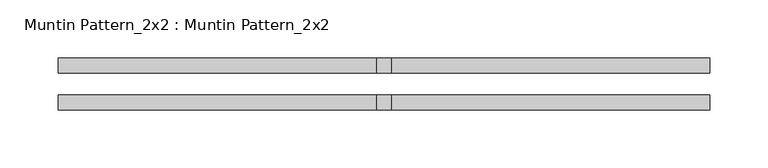
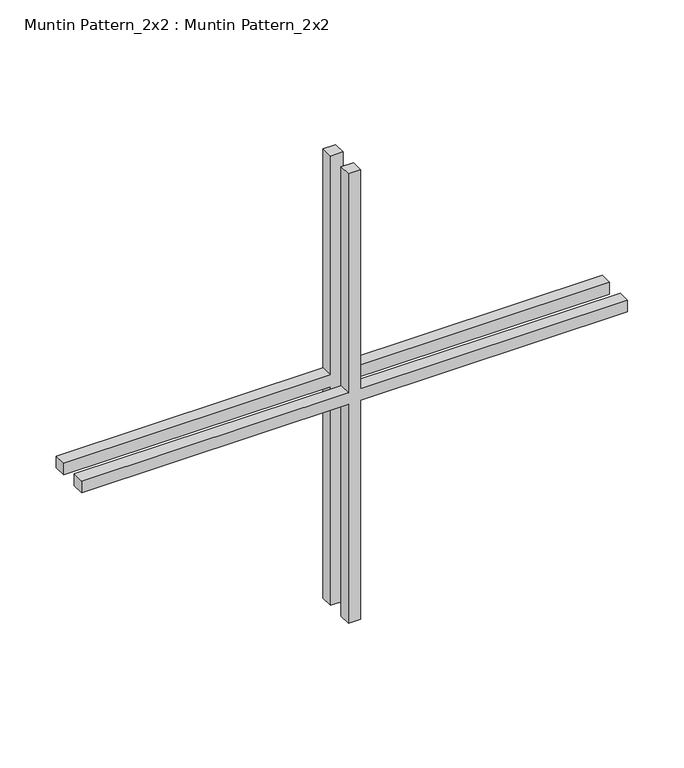
"""IFC4 building model written with IfcOpenShell, lengths in millimetres: proxy geometry, Muntin Pattern_2x2 : Muntin Pattern_2x2."""

from ifc_helpers import new_model, si_unit, frame, origin, place, context, project, spatial, polyline, outline, extrude, source, transform, mapped, element, save


def muntin_pattern_2x2_muntin_pattern_2x2_5f474966(model_context):
    return source(origin(), model_context, "Body", "SweptSolid", [
        extrude(outline(polyline([(249.2375, -6.35), (249.2375, -279.4), (236.5375, -279.4), (236.5375, -6.35), (0.0, -6.35), (0.0, 6.35), (236.5375, 6.35), (236.5375, 279.4), (249.2375, 279.4), (249.2375, 6.35), (485.775, 6.35), (485.775, -6.35), (249.2375, -6.35)])), frame((0.0, 9.525, 0.0), z_axis=(0.0, 1.0, 0.0), x_axis=(0.0, 0.0, 1.0)), (0.0, 0.0, 1.0), 12.7),
        extrude(outline(polyline([(249.2375, -6.35), (249.2375, -279.4), (236.5375, -279.4), (236.5375, -6.35), (0.0, -6.35), (0.0, 6.35), (236.5375, 6.35), (236.5375, 279.4), (249.2375, 279.4), (249.2375, 6.35), (485.775, 6.35), (485.775, -6.35), (249.2375, -6.35)])), frame((0.0, -22.225, 0.0), z_axis=(0.0, 1.0, 0.0), x_axis=(0.0, 0.0, 1.0)), (0.0, 0.0, 1.0), 12.7),
    ])


if __name__ == "__main__":
    model = new_model("IFC4")
    model_context = context("Model", 3, world=origin())
    ifc_project = project(units=[si_unit("LENGTHUNIT", "METRE", prefix="MILLI")], contexts=[model_context])
    site = spatial("IfcSite", under=ifc_project)
    building = spatial("IfcBuilding", under=site)
    placement = place(None, origin())
    muntin_pattern_2x2_muntin_pattern_2x2_shape = muntin_pattern_2x2_muntin_pattern_2x2_5f474966(model_context)
    element("IfcBuildingElementProxy", 1, Name="Muntin Pattern_2x2 : Muntin Pattern_2x2", ObjectType="Muntin Pattern_2x2 : Muntin Pattern_2x2", at=placement, inside=building, context=model_context, shape_type="MappedRepresentation", body=[
        mapped(muntin_pattern_2x2_muntin_pattern_2x2_shape, transform((0.0, 0.0, 0.0), x_axis=(1.0, 0.0, 0.0), y_axis=(0.0, 1.0, 0.0), z_axis=(0.0, 0.0, 1.0))),
    ])
    save(model, "model.ifc")

# Revit data of these elements
# Type "Muntin Pattern_2x2 : Muntin Pattern_2x2"
#   Width [instance default] = 4' - 0"
#   Thickness = 0' - 0 1/2"
#   Height [instance default] = 4' - 0"
#   Distance = 0' - 0 3/4"
#   Interior Material [instance default] = none
#   Exterior Material [instance default] = none
#   Default Elevation = 0
# Element 1 (IfcBuildingElementProxy, "Muntin Pattern_2x2 : Muntin Pattern_2x2")
#   Width = 1' - 10"
#   Height = 1' - 7 1/8"
#   Interior Material = Wood - Stained
#   Exterior Material = Clad - White
#   Materials on its faces: "Clad - White", "Wood - Stained"
# Materials
#   "Clad - White": class "Wood", colour RGB 242 242 238, transparency 0, Cost = 0
#   "Wood - Stained": class "Wood", colour RGB 224 178 126, transparency 0, Cost = 0
